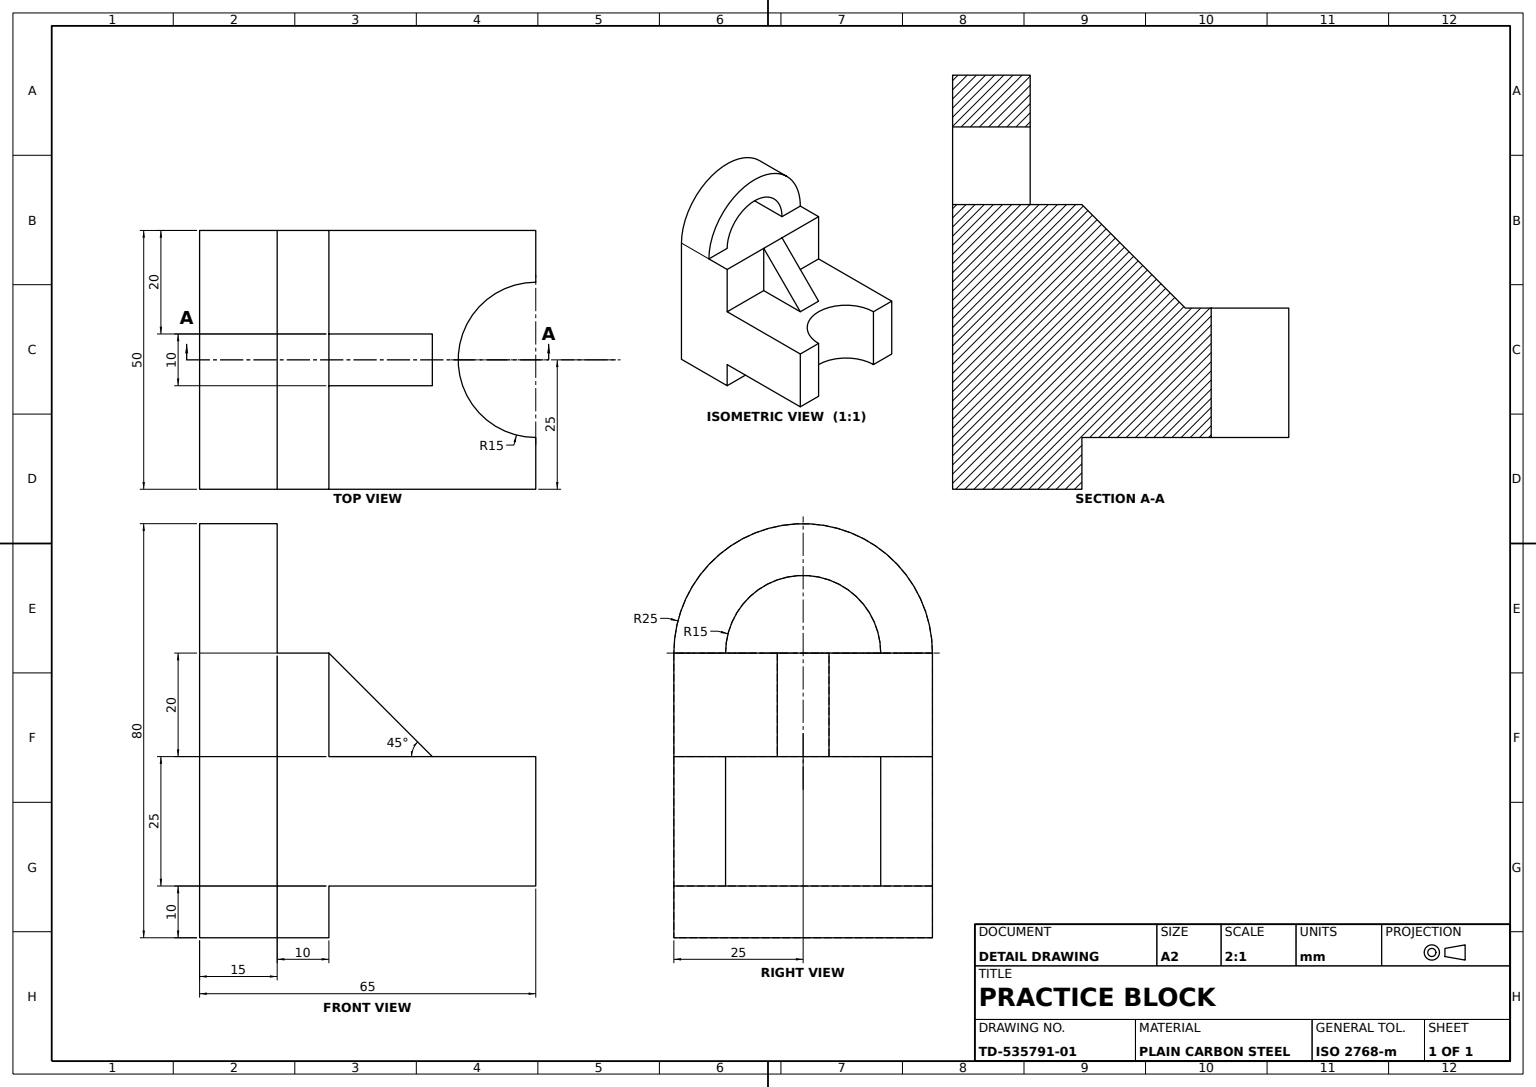
from build123d import *

# Parameters (mm, degrees)
BASE_BLOCK_PROFILE_W      = 65
BASE_BLOCK_PROFILE_H      = 25
BASE_BLOCK_65X25X50_DEPTH = 50
UPRIGHT_PROFILE_W         = 50
UPRIGHT_PROFILE_H         = 20
UPRIGHT_BLOCK_DEPTH       = 25
BOTTOM_TONGUE_PROFILE_W   = 25
BOTTOM_TONGUE_PROFILE_H   = 10
BOTTOM_TONGUE_10X25_DEPTH = 50
END_NOTCH_PROFILE_R       = 15
ROUND_END_NOTCH_DEPTH     = 50
TOP_BOSS_PROFILE_R        = 25
ROUNDED_TOP_BOSS_DEPTH    = 15
BOSS_HALF_HOLE_15_DEPTH   = 15
SUPPORT_WEDGE_DEPTH       = 50
RIB_TRIM_FRONT_DEPTH      = 20
RIB_TRIM_REAR_DEPTH       = 20


with BuildPart() as part:
    # Base Block Profile → Base Block 65x25x50 (new body)
    with BuildSketch(Plane.XY):
        with Locations((32.5, 12.5)):
            Rectangle(BASE_BLOCK_PROFILE_W, BASE_BLOCK_PROFILE_H)
    extrude(amount=-BASE_BLOCK_65X25X50_DEPTH)

    # Upright Profile → Upright Block (add)
    with BuildSketch(Plane.ZY):
        with Locations((-25, 35)):
            Rectangle(UPRIGHT_PROFILE_W, UPRIGHT_PROFILE_H)
    extrude(amount=-UPRIGHT_BLOCK_DEPTH)

    # Bottom Tongue Profile → Bottom Tongue 10x25 (add)
    with BuildSketch(Plane.XY):
        with Locations((12.5, -5)):
            Rectangle(BOTTOM_TONGUE_PROFILE_W, BOTTOM_TONGUE_PROFILE_H)
    extrude(amount=-BOTTOM_TONGUE_10X25_DEPTH)

    # End Notch Profile → Round End Notch (cut)
    with BuildSketch(Plane(origin=(0, 25, 0), x_dir=(1, 0, 0), z_dir=(0, 1, 0))):
        with Locations((65, 25)):
            Circle(END_NOTCH_PROFILE_R)
    extrude(amount=-ROUND_END_NOTCH_DEPTH, mode=Mode.SUBTRACT)

    # Top Boss Profile → Rounded Top Boss (add)
    with BuildSketch(Plane.ZY):
        with Locations((-25, 45)):
            Circle(TOP_BOSS_PROFILE_R)
    extrude(amount=-ROUNDED_TOP_BOSS_DEPTH)

    # Boss Hole Profile → Boss Half Hole Ø15 (cut)
    with BuildSketch(Plane(origin=(15, 0, 0), x_dir=(0, 0, -1), z_dir=(1, 0, 0))):
        with BuildLine():
            Line((10, 45), (40, 45))
            ThreePointArc((40, 45), (25, 60), (10, 45))
        make_face()
    extrude(amount=-BOSS_HALF_HOLE_15_DEPTH, mode=Mode.SUBTRACT)

    # Support Wedge Profile → Support Wedge (add)
    with BuildSketch(Plane.XY):
        Polygon((25, 45), (25, 25), (45, 25), align=None)
    extrude(amount=-SUPPORT_WEDGE_DEPTH)

    # Rib Trim Front Profile → Rib Trim Front (cut)
    with BuildSketch(Plane.XY):
        Polygon((25, 45), (45, 25), (25, 25), align=None)
    extrude(amount=-RIB_TRIM_FRONT_DEPTH, mode=Mode.SUBTRACT)

    # Rib Trim Rear Profile → Rib Trim Rear (cut)
    with BuildSketch(Plane(origin=(0, 0, -50), x_dir=(-1, 0, 0), z_dir=(0, 0, -1))):
        Polygon((-25, 45), (-25, 25), (-45, 25), align=None)
    extrude(amount=-RIB_TRIM_REAR_DEPTH, mode=Mode.SUBTRACT)


solid = part.part
